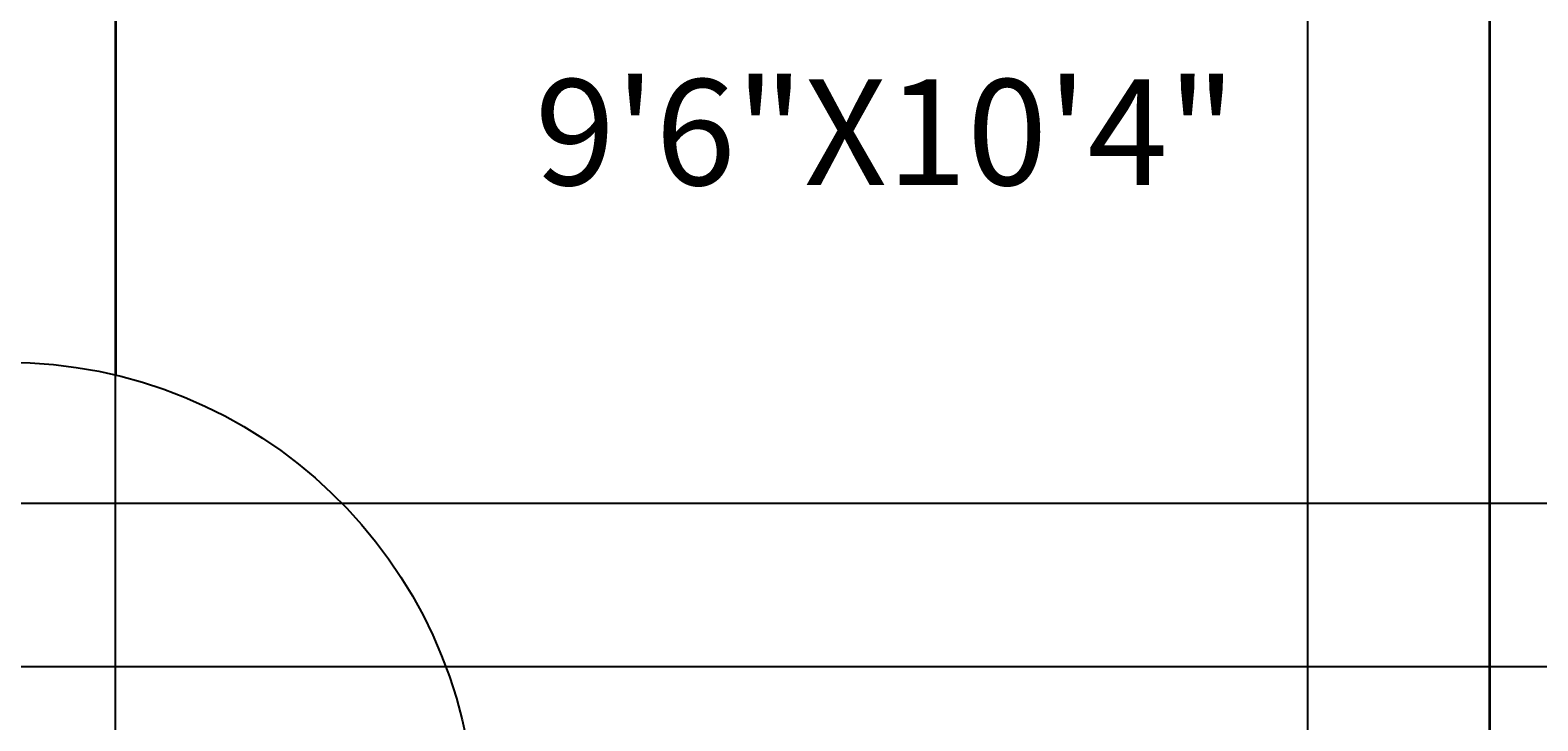
# Model space of a CAD drawing. Units: feet. Extents: x 100807 to 101423, y 154875 to 156331.
# Tile 4 of 8: x 101051 to 101176, y 156040 to 156097. Entities that reach past the tile are written whole.
import ezdxf

# ---------------------------------------------------------------- set-up
doc = ezdxf.new("R2010")
doc.units = ezdxf.units.FT
for name, color, linetype, lineweight in [('A-ANNO-DIMS', 2, 'Continuous', 18), ('A-DOOR', 4, 'Continuous', 25), ('A-WALL', 7, 'Continuous', 35)]:
    doc.layers.add(name, color=color, linetype=linetype, lineweight=lineweight)
doc.styles.get("Standard").update_dxf_attribs({"font": 'arial.ttf'})
doc.dimstyles.get("Standard").update_dxf_attribs({"dimtxt": 0.18, "dimasz": 0.18, "dimexe": 0.18, "dimexo": 0.0625, "dimgap": 0.09, "dimtad": 0, "dimtih": 1, "dimtoh": 1, "dimdec": 4, "dimzin": 0, "dimdsep": 46, "dimtxsty": 'Standard', "dimcen": 0.09, "dimadec": 0, "dimazin": 0, "dimtfac": 1, "dimtdec": 4, "dimtofl": 0, "dimtmove": 0, "dimatfit": 3, "dimfxl": 1, "dimtolj": 1, "dimtzin": 0, "dimarcsym": 0})

# ---------------------------------------------------------------- blocks, each defined once
blk = doc.blocks.new('DR-36')
for p, q in [((0, 36), (0, 0)), ((0, 36), (1.5, 36)), ((1.5, 36), (1.5, 0)), ((0, 0), (1.5, 0))]:
    blk.add_line(p, q)
blk.add_arc((0, 0), 36, 0, 87.6141)
blk = doc.blocks.new('*D36')
at = {"layer": 'A-ANNO-DIMS', "color": 0, "lineweight": -2, "transparency": 16777216}
for p, q in [((101058.16, 155866.64), (101058.16, 156302.91)), ((101058.34, 156302.73), (101114.88, 156302.73)), ((101171.98, 156302.73), (101115.44, 156302.73)), ((101172.16, 155866.64), (101172.16, 156302.91))]:
    blk.add_line(p, q, dxfattribs=at)
at = {"layer": 'A-ANNO-DIMS', "color": 0, "transparency": 16777216}
for points in [[(101058.34, 156302.76), (101058.34, 156302.7), (101058.16, 156302.73)], [(101171.98, 156302.76), (101171.98, 156302.7), (101172.16, 156302.73)]]:
    blk.add_solid(points, dxfattribs=at)
at = {"layer": 'Defpoints', "color": 0, "transparency": 16777216}
for p in [(101172.16, 156302.73), (101058.16, 155866.58), (101172.16, 155866.58)]:
    blk.add_point(p, dxfattribs=at)
at = {"layer": 'A-ANNO-DIMS', "color": 0, "transparency": 16777216, "insert": (101115.16, 156302.73), "char_height": 0.18, "attachment_point": 5}
blk.add_mtext('\\A1;114', dxfattribs=at)
blk = doc.blocks.new('*D49')
at = {"layer": 'A-ANNO-DIMS', "color": 0, "lineweight": -2, "transparency": 16777216}
for p, q in [((101157.08, 155866.64), (101157.08, 156302.91)), ((101157.26, 156302.73), (101164.16, 156302.73)), ((101171.98, 156302.73), (101165.07, 156302.73)), ((101172.16, 155866.64), (101172.16, 156302.91))]:
    blk.add_line(p, q, dxfattribs=at)
at = {"layer": 'A-ANNO-DIMS', "color": 0, "transparency": 16777216}
for points in [[(101157.26, 156302.76), (101157.26, 156302.7), (101157.08, 156302.73)], [(101171.98, 156302.76), (101171.98, 156302.7), (101172.16, 156302.73)]]:
    blk.add_solid(points, dxfattribs=at)
at = {"layer": 'Defpoints', "color": 0, "transparency": 16777216}
for p in [(101172.16, 156302.73), (101157.08, 155866.58), (101172.16, 155866.58)]:
    blk.add_point(p, dxfattribs=at)
at = {"layer": 'A-ANNO-DIMS', "color": 0, "transparency": 16777216, "insert": (101164.62, 156302.73), "char_height": 0.18, "attachment_point": 5}
blk.add_mtext('\\A1;15.075', dxfattribs=at)
blk = doc.blocks.new('*D55')
at = {"layer": 'A-ANNO-DIMS', "color": 0, "lineweight": -2, "transparency": 16777216}
for p, q in [((100908.22, 156058.13), (101422.49, 156058.13)), ((101422.31, 156057.95), (101422.31, 156051.53)), ((101422.31, 156044.76), (101422.31, 156051.17)), ((100908.22, 156044.58), (101422.49, 156044.58))]:
    blk.add_line(p, q, dxfattribs=at)
at = {"layer": 'A-ANNO-DIMS', "color": 0, "transparency": 16777216}
for points in [[(101422.28, 156057.95), (101422.34, 156057.95), (101422.31, 156058.13)], [(101422.28, 156044.76), (101422.34, 156044.76), (101422.31, 156044.58)]]:
    blk.add_solid(points, dxfattribs=at)
at = {"layer": 'Defpoints', "color": 0, "transparency": 16777216}
for p in [(100908.16, 156058.13), (101422.31, 156058.13), (100908.16, 156044.58)]:
    blk.add_point(p, dxfattribs=at)
at = {"layer": 'A-ANNO-DIMS', "color": 0, "transparency": 16777216, "insert": (101422.31, 156051.35), "char_height": 0.18, "attachment_point": 5}
blk.add_mtext('\\A1;13.55', dxfattribs=at)

msp = doc.modelspace()

# ---------------------------------------------------------------- linework, layer by layer
at = {"layer": 'A-WALL'}
for p, q in [((101058.1564, 156156.5789), (101058.1564, 156068.7713)), ((101172.1564, 156156.5789), (101172.1564, 156032.5789))]:
    msp.add_line(p, q, dxfattribs=at)

# ---------------------------------------------------------------- block references
at = {"layer": 'A-DOOR', "xscale": -1.079672442471032, "yscale": 1.079672442471032, "zscale": 1.079672442471032, "rotation": 270.0000000000369}
msp.add_blockref('DR-36', (101049.1564, 156030.9594), dxfattribs=at)

# ---------------------------------------------------------------- texts
at = {"layer": 'A-ANNO-DIMS'}
msp.add_text('9\'6"X10\'4"', height=8.78822, dxfattribs=at).set_placement((101092.9589, 156084.5286))

# ---------------------------------------------------------------- dimensions: what is measured, and where the dimension line sits
for p1, override, picture, middle in [((101058.1564, 155866.5789), {"dimdec": 0, "dimlfac": 1, "dimrnd": 0, "dimzin": 0, "dimdsep": 46, "dimlunit": 2}, '*D36', (101115.1564, 156302.7277)), ((101157.0816, 155866.5789), {"dimdec": 3, "dimlfac": 1, "dimrnd": 0, "dimzin": 0, "dimdsep": 46, "dimlunit": 2}, '*D49', (101164.619, 156302.7277))]:
    dim = msp.add_linear_dim(base=(101172.1564, 156302.7277), p1=p1, p2=(101172.1564, 155866.5789), dimstyle='Standard', override=override, dxfattribs=at)
    dim.commit()
    dim.dimension.update_dxf_attribs({"geometry": picture, "text_midpoint": middle})
dim = msp.add_linear_dim(base=(101422.3064, 156058.1276), p1=(100908.1564, 156044.5777), p2=(100908.1564, 156058.1276), angle=90, dimstyle='Standard', override={"dimdec": 2, "dimlfac": 1, "dimrnd": 0, "dimzin": 0, "dimdsep": 46, "dimlunit": 2}, dxfattribs=at)
dim.commit()
dim.dimension.update_dxf_attribs({"geometry": '*D55', "text_midpoint": (101422.3064, 156051.3527)})

doc.saveas('drawing.dxf')
